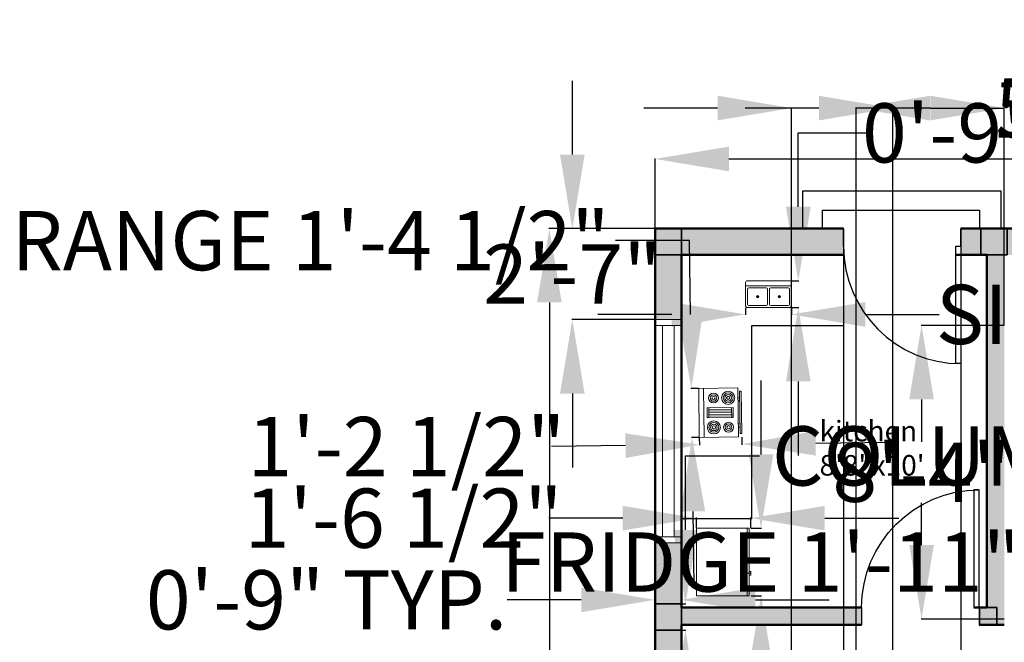
# Model space of a CAD drawing. Units: inches. Extents: x 25 to 82118, y 10 to 6494.
# Tile 2 of 9: x 40498 to 40833, y 3391 to 3603. Entities that reach past the tile are written whole.
import ezdxf

# ---------------------------------------------------------------- set-up
doc = ezdxf.new("R2010")
doc.units = ezdxf.units.IN
doc.header["$MEASUREMENT"] = 0
for name, color, linetype, lineweight in [('A-ANNO-DIMS', 2, 'Continuous', 18), ('A-AREA-IDEN', 7, 'Continuous', 25), ('A-DOOR', 3, 'Continuous', 25), ('A-EQPM', 8, 'Continuous', 18), ('A-FLOR-CASE', 8, 'Continuous', 25), ('A-FLOR-FIXT', 9, 'Continuous', 18), ('A-FLOR-STRS', 7, 'Continuous', 25), ('A-GLAZ', 4, 'Continuous', 18), ('A-WALL', 7, 'Continuous', 50)]:
    doc.layers.add(name, color=color, linetype=linetype, lineweight=lineweight)
doc.layers.add('A-COLS', color=30, linetype='Continuous', lineweight=35, true_color=0xf26722)
doc.layers.add('A-WALL-PATT', color=18, linetype='Continuous', lineweight=13, true_color=0x000000)
doc.styles.get("Standard").update_dxf_attribs({"font": 'arial.ttf'})
doc.dimstyles.get("Standard").update_dxf_attribs({"dimtxt": 20.18, "dimasz": 25.18, "dimexe": 0.18, "dimexo": 0.0625, "dimgap": 0.09, "dimtad": 0, "dimtih": 1, "dimtoh": 1, "dimdec": 0, "dimzin": 0, "dimdsep": 46, "dimlunit": 3, "dimtxsty": 'Standard', "dimcen": 0.09, "dimadec": 0, "dimazin": 0, "dimtfac": 1, "dimtdec": 0, "dimtofl": 0, "dimtmove": 0, "dimatfit": 3, "dimfxl": 1, "dimtolj": 1, "dimtzin": 0, "dimarcsym": 0})

# ---------------------------------------------------------------- blocks, each defined once
blk = doc.blocks.new('Sink-double - 36 in top')
for p, q in [((-18, -4), (18, -4)), ((-0.75, -18.5), (-0.75, -6.5)), ((0.75, -6.5), (0.75, -18.5))]:
    blk.add_line(p, q)
for points in [[(-16.5, 0), (16.5, 0)], [(-18, -19.5), (-18, -1.5)], [(-16.5, -18.5), (-16.5, -6.5)], [(-15.5, -5.5), (-1.75, -5.5)], [(1.75, -5.5), (15.5, -5.5)], [(16.5, -6.5), (16.5, -18.5)], [(18, -1.5), (18, -19.5)], [(16.5, -21), (-16.5, -21)], [(-1.75, -19.5), (-15.5, -19.5)], [(15.5, -19.5), (1.75, -19.5)]]:
    blk.add_lwpolyline(points)
for centre, radius in [((-8.5, -12.5), 1), ((-8.5, -12.5), 0.5), ((8.5, -12.5), 1), ((8.5, -12.5), 0.5)]:
    blk.add_circle(centre, radius)
for centre, radius, start, end in [((-16.5, -1.5), 1.5, 90, 180), ((16.5, -1.5), 1.5, 0, 90), ((-15.5, -6.5), 1, 90, 180), ((-1.75, -6.5), 1, 0, 90), ((1.75, -6.5), 1, 90, 180), ((15.5, -6.5), 1, 0, 90), ((-16.5, -19.5), 1.5, 180, 270), ((-15.5, -18.5), 1, 180, 270), ((-1.75, -18.5), 1, 270, 0), ((1.75, -18.5), 1, 180, 270), ((15.5, -18.5), 1, 270, 0), ((16.5, -19.5), 1.5, 270, 0)]:
    blk.add_arc(centre, radius, start, end)
blk = doc.blocks.new('Range-Oven - 30 in top')
for p, q in [((0, -3), (30, -3)), ((12, -6), (18, -6)), ((13, -20), (13, -6)), ((14, -6), (14, -20)), ((15, -20), (15, -6)), ((16, -6), (16, -20)), ((17, -20), (17, -6)), ((6, -24), (6, -25)), ((8, -25), (8, -24)), ((18, -20), (12, -20)), ((22, -25), (22, -24)), ((24, -24), (24, -25))]:
    blk.add_line(p, q)
for points in [[(0, -24), (0, 0), (30, 0), (30, -24)], [(12, -21), (12, -5), (18, -5), (18, -21)], [(2, -26), (2, -25), (28, -25), (28, -26)]]:
    blk.add_lwpolyline(points, close=True)
for centre, radius in [((6, -9), 4), ((6, -9), 3), ((24, -9), 3), ((6, -9), 2), ((6, -9), 1), ((24, -9), 2), ((24, -9), 1), ((6, -18), 3), ((6, -18), 2), ((6, -18), 1), ((24, -18), 4), ((24, -18), 3), ((24, -18), 2), ((24, -18), 1)]:
    blk.add_circle(centre, radius)
blk = doc.blocks.new('*U12')
for p, q in [((0, 0), (0, -6)), ((40, 0), (40, -6))]:
    blk.add_line(p, q)
blk.add_lwpolyline([(0, 0), (0, 40), (1.75, 40), (1.75, 0)], close=True)
blk.add_arc((0, 0), 40, 0, 90)
blk = doc.blocks.new('Refrigerator-2 door - 36 in top')
for p, q in [((0, -26.999999), (36, -26.999999)), ((11, -27.999999), (11, -28.999999)), ((11, -28.999999), (13, -28.999999)), ((12, -26.999999), (12, -28.999999)), ((13, -28.999999), (13, -27.999999))]:
    blk.add_line(p, q)
blk.add_lwpolyline([(0, -27.999999), (0, 0), (36, 0), (36, -27.999999)], close=True)
blk = doc.blocks.new('*D13')
at = {"layer": 'A-ANNO-DIMS', "color": 0, "lineweight": -2, "transparency": 16777216}
for p, q in [((40714.21, 3531.88), (40714.21, 3555.71)), ((40739.39, 3555.53), (40877, 3555.53)), ((41049.03, 3555.53), (40911.42, 3555.53)), ((41074.21, 3531.88), (41074.21, 3555.71))]:
    blk.add_line(p, q, dxfattribs=at)
at = {"layer": 'A-ANNO-DIMS', "color": 0, "transparency": 16777216}
for points in [[(40739.39, 3559.72), (40739.39, 3551.33), (40714.21, 3555.53)], [(41049.03, 3559.72), (41049.03, 3551.33), (41074.21, 3555.53)]]:
    blk.add_solid(points, dxfattribs=at)
at = {"layer": 'Defpoints', "color": 0, "transparency": 16777216}
for p in [(41074.21, 3555.53), (40714.21, 3531.82), (41074.21, 3531.82)]:
    blk.add_point(p, dxfattribs=at)
at = {"layer": 'A-ANNO-DIMS', "color": 0, "transparency": 16777216, "insert": (40894.21, 3555.53), "char_height": 20.18, "attachment_point": 5}
blk.add_mtext("\\A1;30'", dxfattribs=at)
blk = doc.blocks.new('*D14')
at = {"layer": 'A-ANNO-DIMS', "color": 0, "lineweight": -2, "transparency": 16777216}
for p, q in [((40714.15, 3531.82), (40678.01, 3531.82)), ((40678.19, 3506.64), (40678.19, 3350.2)), ((40678.19, 3172.97), (40678.19, 3329.4)), ((40714.15, 3147.79), (40678.01, 3147.79))]:
    blk.add_line(p, q, dxfattribs=at)
at = {"layer": 'A-ANNO-DIMS', "color": 0, "transparency": 16777216}
for points in [[(40673.99, 3506.64), (40682.39, 3506.64), (40678.19, 3531.82)], [(40673.99, 3172.97), (40682.39, 3172.97), (40678.19, 3147.79)]]:
    blk.add_solid(points, dxfattribs=at)
at = {"layer": 'Defpoints', "color": 0, "transparency": 16777216}
for p in [(40714.21, 3531.82), (40678.19, 3147.79), (40714.21, 3147.79)]:
    blk.add_point(p, dxfattribs=at)
at = {"layer": 'A-ANNO-DIMS', "color": 0, "transparency": 16777216, "insert": (40678.19, 3339.8), "char_height": 20.18, "attachment_point": 5}
blk.add_mtext("\\A1;32'", dxfattribs=at)
blk = doc.blocks.new('WIN-72IN-9W')
for p, q in [((9, 76), (0, 76)), ((9, 74), (0, 74)), ((2.5, 74), (2.5, 2)), ((6.5, 74), (6.5, 2)), ((9, 2), (0, 2)), ((9, 0), (0, 0))]:
    blk.add_line(p, q)
blk = doc.blocks.new('COL-9X9')
h = blk.add_hatch(color=256)
h.dxf.hatch_style = 1
h.paths.add_polyline_path([(9, 9), (0, 9), (0, 0), (9, 0)])
blk.add_lwpolyline([(0, 0), (9, 0), (9, 9), (0, 9)], close=True)
blk = doc.blocks.new('POST-INTERIOR-6IN')
h = blk.add_hatch(color=256)
h.dxf.hatch_style = 1
h.paths.add_polyline_path([(6, 5.8), (0, 5.8), (0, 0), (6, 0)])
blk.add_lwpolyline([(6, 5.8), (0, 5.8), (0, 0), (6, 0)], close=True)
blk = doc.blocks.new('*D25')
at = {"layer": 'A-ANNO-DIMS', "color": 0, "lineweight": -2, "transparency": 16777216}
for p, q in [((40724.56, 3429.21), (40724.56, 3454.39)), ((40724.56, 3454.39), (40749.74, 3454.39)), ((40723.27, 3404.03), (40724.74, 3404.03)), ((40723.27, 3395.03), (40724.74, 3395.03)), ((40724.56, 3369.85), (40724.56, 3344.67))]:
    blk.add_line(p, q, dxfattribs=at)
at = {"layer": 'A-ANNO-DIMS', "color": 0, "transparency": 16777216}
for points in [[(40720.36, 3429.21), (40728.76, 3429.21), (40724.56, 3404.03)], [(40720.36, 3369.85), (40728.76, 3369.85), (40724.56, 3395.03)]]:
    blk.add_solid(points, dxfattribs=at)
at = {"layer": 'Defpoints', "color": 0, "transparency": 16777216}
for p in [(40723.21, 3404.03), (40724.56, 3404.03), (40723.21, 3395.03)]:
    blk.add_point(p, dxfattribs=at)
at = {"layer": 'A-ANNO-DIMS', "color": 0, "transparency": 16777216, "insert": (40876.22, 3454.39), "char_height": 20.18, "attachment_point": 5}
blk.add_mtext('\\A1;COLUMN 0\'-9" TYP.', dxfattribs=at)
blk = doc.blocks.new('*D26')
at = {"layer": 'A-ANNO-DIMS', "color": 0, "lineweight": -2, "transparency": 16777216}
for p, q in [((40714.21, 3404.09), (40714.21, 3405.56)), ((40723.21, 3404.09), (40723.21, 3405.56)), ((40689.03, 3405.38), (40663.85, 3405.38)), ((40748.39, 3405.38), (40773.57, 3405.38))]:
    blk.add_line(p, q, dxfattribs=at)
at = {"layer": 'A-ANNO-DIMS', "color": 0, "transparency": 16777216}
for points in [[(40689.03, 3409.57), (40689.03, 3401.18), (40714.21, 3405.38)], [(40748.39, 3409.57), (40748.39, 3401.18), (40723.21, 3405.38)]]:
    blk.add_solid(points, dxfattribs=at)
at = {"layer": 'Defpoints', "color": 0, "transparency": 16777216}
for p in [(40714.21, 3405.38), (40714.21, 3404.03), (40723.21, 3404.03)]:
    blk.add_point(p, dxfattribs=at)
at = {"layer": 'A-ANNO-DIMS', "color": 0, "transparency": 16777216, "insert": (40602.26, 3405.38), "char_height": 20.18, "attachment_point": 5}
blk.add_mtext('\\A1;0\'-9" TYP.', dxfattribs=at)
blk = doc.blocks.new('*D37')
at = {"layer": 'A-ANNO-DIMS', "color": 0, "lineweight": -2, "transparency": 16777216}
for p, q in [((40745.04, 3504.86), (40745.04, 3502.4)), ((40760.67, 3504.86), (40760.67, 3502.4)), ((40719.86, 3502.58), (40694.68, 3502.58)), ((40785.85, 3502.58), (40811.03, 3502.58))]:
    blk.add_line(p, q, dxfattribs=at)
at = {"layer": 'A-ANNO-DIMS', "color": 0, "transparency": 16777216}
for points in [[(40719.86, 3506.78), (40719.86, 3498.38), (40745.04, 3502.58)], [(40785.85, 3506.78), (40785.85, 3498.38), (40760.67, 3502.58)]]:
    blk.add_solid(points, dxfattribs=at)
at = {"layer": 'Defpoints', "color": 0, "transparency": 16777216}
for p in [(40745.04, 3504.92), (40760.67, 3504.92), (40760.67, 3502.58)]:
    blk.add_point(p, dxfattribs=at)
at = {"layer": 'A-ANNO-DIMS', "color": 0, "transparency": 16777216, "insert": (40898.22, 3502.58), "char_height": 20.18, "attachment_point": 5}
blk.add_mtext('\\A1;SINK 1\'-3 1/2"', dxfattribs=at)
blk = doc.blocks.new('*D38')
at = {"layer": 'A-ANNO-DIMS', "color": 0, "lineweight": -2, "transparency": 16777216}
for p, q in [((40763.01, 3539.22), (40763.01, 3564.4)), ((40763.01, 3564.4), (40788.19, 3564.4)), ((40760.73, 3514.04), (40763.19, 3514.04)), ((40760.73, 3504.92), (40763.19, 3504.92)), ((40763.01, 3479.74), (40763.01, 3454.56))]:
    blk.add_line(p, q, dxfattribs=at)
at = {"layer": 'A-ANNO-DIMS', "color": 0, "transparency": 16777216}
for points in [[(40758.81, 3539.22), (40767.21, 3539.22), (40763.01, 3514.04)], [(40758.81, 3479.74), (40767.21, 3479.74), (40763.01, 3504.92)]]:
    blk.add_solid(points, dxfattribs=at)
at = {"layer": 'Defpoints', "color": 0, "transparency": 16777216}
for p in [(40760.67, 3514.04), (40763.01, 3514.04), (40760.67, 3504.92)]:
    blk.add_point(p, dxfattribs=at)
at = {"layer": 'A-ANNO-DIMS', "color": 0, "transparency": 16777216, "insert": (40815.1, 3564.4), "char_height": 20.18, "attachment_point": 5}
blk.add_mtext('\\A1;0\'-9"', dxfattribs=at)
blk = doc.blocks.new('*D39')
at = {"layer": 'A-ANNO-DIMS', "color": 0, "lineweight": -2, "transparency": 16777216}
for p, q in [((40725.94, 3527.71), (40700.76, 3527.71)), ((40726.26, 3502.53), (40725.94, 3527.71)), ((40729.01, 3477.38), (40726.39, 3477.35)), ((40729.22, 3460.71), (40726.6, 3460.68)), ((40727.1, 3435.5), (40727.41, 3410.32))]:
    blk.add_line(p, q, dxfattribs=at)
at = {"layer": 'A-ANNO-DIMS', "color": 0, "transparency": 16777216}
for points in [[(40730.45, 3502.58), (40722.06, 3502.48), (40726.57, 3477.35)], [(40731.29, 3435.55), (40722.9, 3435.45), (40726.78, 3460.68)]]:
    blk.add_solid(points, dxfattribs=at)
at = {"layer": 'Defpoints', "color": 0, "transparency": 16777216}
for p in [(40726.57, 3477.35), (40729.07, 3477.38), (40729.28, 3460.71)]:
    blk.add_point(p, dxfattribs=at)
at = {"layer": 'A-ANNO-DIMS', "color": 0, "transparency": 16777216, "insert": (40596.82, 3527.71), "char_height": 20.18, "attachment_point": 5}
blk.add_mtext('\\A1;RANGE 1\'-4 1/2"', dxfattribs=at)
blk = doc.blocks.new('*D40')
at = {"layer": 'A-ANNO-DIMS', "color": 0, "lineweight": -2, "transparency": 16777216}
for p, q in [((40729.28, 3460.65), (40729.32, 3458.03)), ((40743.73, 3460.83), (40743.76, 3458.21)), ((40704.14, 3457.89), (40678.96, 3457.58)), ((40768.94, 3458.71), (40794.12, 3459.02))]:
    blk.add_line(p, q, dxfattribs=at)
at = {"layer": 'A-ANNO-DIMS', "color": 0, "transparency": 16777216}
for points in [[(40768.89, 3462.9), (40768.99, 3454.51), (40743.76, 3458.39)], [(40704.08, 3462.09), (40704.19, 3453.7), (40729.31, 3458.21)]]:
    blk.add_solid(points, dxfattribs=at)
at = {"layer": 'Defpoints', "color": 0, "transparency": 16777216}
for p in [(40729.28, 3460.71), (40743.73, 3460.89), (40729.31, 3458.21)]:
    blk.add_point(p, dxfattribs=at)
at = {"layer": 'A-ANNO-DIMS', "color": 0, "transparency": 16777216, "insert": (40629.48, 3457.58), "char_height": 20.18, "attachment_point": 5}
blk.add_mtext('\\A1;1\'-2 1/2"', dxfattribs=at)
blk = doc.blocks.new('*D51')
at = {"layer": 'A-ANNO-DIMS', "color": 0, "lineweight": -2, "transparency": 16777216}
for p, q in [((40750.31, 3454.92), (40750.31, 3480.1)), ((40746.92, 3429.74), (40750.49, 3429.74)), ((40746.92, 3406.76), (40750.49, 3406.76)), ((40750.31, 3381.58), (40750.31, 3356.4))]:
    blk.add_line(p, q, dxfattribs=at)
at = {"layer": 'A-ANNO-DIMS', "color": 0, "transparency": 16777216}
for points in [[(40746.11, 3454.92), (40754.5, 3454.92), (40750.31, 3429.74)], [(40746.11, 3381.58), (40754.5, 3381.58), (40750.31, 3406.76)]]:
    blk.add_solid(points, dxfattribs=at)
at = {"layer": 'Defpoints', "color": 0, "transparency": 16777216}
for p in [(40746.86, 3429.74), (40750.31, 3429.74), (40746.86, 3406.76)]:
    blk.add_point(p, dxfattribs=at)
at = {"layer": 'A-ANNO-DIMS', "color": 0, "transparency": 16777216, "insert": (40750.31, 3418.25), "char_height": 20.18, "attachment_point": 5}
blk.add_mtext('\\A1;FRIDGE 1\'-11"', dxfattribs=at)
blk = doc.blocks.new('*D52')
at = {"layer": 'A-ANNO-DIMS', "color": 0, "lineweight": -2, "transparency": 16777216}
for p, q in [((40703.17, 3433.19), (40677.99, 3433.19)), ((40728.35, 3429.8), (40728.35, 3433.37)), ((40746.86, 3429.8), (40746.86, 3433.37)), ((40772.04, 3433.19), (40797.22, 3433.19))]:
    blk.add_line(p, q, dxfattribs=at)
at = {"layer": 'A-ANNO-DIMS', "color": 0, "transparency": 16777216}
for points in [[(40703.17, 3437.39), (40703.17, 3428.99), (40728.35, 3433.19)], [(40772.04, 3437.39), (40772.04, 3428.99), (40746.86, 3433.19)]]:
    blk.add_solid(points, dxfattribs=at)
at = {"layer": 'Defpoints', "color": 0, "transparency": 16777216}
for p in [(40728.35, 3433.19), (40728.35, 3429.74), (40746.86, 3429.74)]:
    blk.add_point(p, dxfattribs=at)
at = {"layer": 'A-ANNO-DIMS', "color": 0, "transparency": 16777216, "insert": (40628.52, 3433.19), "char_height": 20.18, "attachment_point": 5}
blk.add_mtext('\\A1;1\'-6 1/2"', dxfattribs=at)
blk = doc.blocks.new('*D53')
at = {"layer": 'A-ANNO-DIMS', "color": 0, "lineweight": -2, "transparency": 16777216}
for p, q in [((40808.03, 3572.85), (40782.85, 3572.85)), ((40833.21, 3498.88), (40833.21, 3573.03)), ((40903.21, 3498.88), (40903.21, 3573.03)), ((40928.39, 3572.85), (40953.57, 3572.85))]:
    blk.add_line(p, q, dxfattribs=at)
at = {"layer": 'A-ANNO-DIMS', "color": 0, "transparency": 16777216}
for points in [[(40808.03, 3577.05), (40808.03, 3568.66), (40833.21, 3572.85)], [(40928.39, 3577.05), (40928.39, 3568.66), (40903.21, 3572.85)]]:
    blk.add_solid(points, dxfattribs=at)
at = {"layer": 'Defpoints', "color": 0, "transparency": 16777216}
for p in [(40903.21, 3572.85), (40833.21, 3498.82), (40903.21, 3498.82)]:
    blk.add_point(p, dxfattribs=at)
at = {"layer": 'A-ANNO-DIMS', "color": 0, "transparency": 16777216, "insert": (40868.21, 3572.85), "char_height": 20.18, "attachment_point": 5}
blk.add_mtext('\\A1;5\'-10"', dxfattribs=at)
blk = doc.blocks.new('*D54')
at = {"layer": 'A-ANNO-DIMS', "color": 0, "lineweight": -2, "transparency": 16777216}
for p, q in [((40833.15, 3498.82), (40804.83, 3498.82)), ((40805.01, 3473.64), (40805.01, 3459.21)), ((40805.01, 3424), (40805.01, 3438.43)), ((40833.15, 3398.82), (40804.83, 3398.82))]:
    blk.add_line(p, q, dxfattribs=at)
at = {"layer": 'A-ANNO-DIMS', "color": 0, "transparency": 16777216}
for points in [[(40800.81, 3473.64), (40809.21, 3473.64), (40805.01, 3498.82)], [(40800.81, 3424), (40809.21, 3424), (40805.01, 3398.82)]]:
    blk.add_solid(points, dxfattribs=at)
at = {"layer": 'Defpoints', "color": 0, "transparency": 16777216}
for p in [(40805.01, 3498.82), (40833.21, 3498.82), (40833.21, 3398.82)]:
    blk.add_point(p, dxfattribs=at)
at = {"layer": 'A-ANNO-DIMS', "color": 0, "transparency": 16777216, "insert": (40805.01, 3448.82), "char_height": 20.18, "attachment_point": 5}
blk.add_mtext('\\A1;8\'-4"', dxfattribs=at)
blk = doc.blocks.new('*D56')
at = {"layer": 'A-ANNO-DIMS', "color": 0, "lineweight": -2, "transparency": 16777216}
for p, q in [((40778.43, 3531.76), (40778.43, 3119.41)), ((40818.43, 3531.76), (40818.43, 3119.41)), ((40753.25, 3119.59), (40728.07, 3119.59)), ((40843.61, 3119.59), (40868.79, 3119.59))]:
    blk.add_line(p, q, dxfattribs=at)
at = {"layer": 'A-ANNO-DIMS', "color": 0, "transparency": 16777216}
for points in [[(40753.25, 3123.78), (40753.25, 3115.39), (40778.43, 3119.59)], [(40843.61, 3123.78), (40843.61, 3115.39), (40818.43, 3119.59)]]:
    blk.add_solid(points, dxfattribs=at)
at = {"layer": 'Defpoints', "color": 0, "transparency": 16777216}
for p in [(40778.43, 3531.82), (40818.43, 3531.82), (40818.43, 3119.59)]:
    blk.add_point(p, dxfattribs=at)
at = {"layer": 'A-ANNO-DIMS', "color": 0, "transparency": 16777216, "insert": (40895.69, 3119.59), "char_height": 20.18, "attachment_point": 5}
blk.add_mtext('\\A1;3\'-4"', dxfattribs=at)
blk = doc.blocks.new('*D57')
at = {"layer": 'A-ANNO-DIMS', "color": 0, "lineweight": -2, "transparency": 16777216}
for p, q in [((40714.21, 3531.76), (40714.21, 3119.41)), ((40778.43, 3531.76), (40778.43, 3119.41)), ((40689.03, 3119.59), (40663.85, 3119.59)), ((40803.61, 3119.59), (40828.79, 3119.59))]:
    blk.add_line(p, q, dxfattribs=at)
at = {"layer": 'A-ANNO-DIMS', "color": 0, "transparency": 16777216}
for points in [[(40689.03, 3123.78), (40689.03, 3115.39), (40714.21, 3119.59)], [(40803.61, 3123.78), (40803.61, 3115.39), (40778.43, 3119.59)]]:
    blk.add_solid(points, dxfattribs=at)
at = {"layer": 'Defpoints', "color": 0, "transparency": 16777216}
for p in [(40714.21, 3531.82), (40778.43, 3531.82), (40778.43, 3119.59)]:
    blk.add_point(p, dxfattribs=at)
at = {"layer": 'A-ANNO-DIMS', "color": 0, "transparency": 16777216, "insert": (40746.32, 3119.59), "char_height": 20.18, "attachment_point": 5}
blk.add_mtext('\\A1;5\'-4"', dxfattribs=at)
blk = doc.blocks.new('*D58')
at = {"layer": 'A-ANNO-DIMS', "color": 0, "lineweight": -2, "transparency": 16777216}
for p, q in [((40735.53, 3572.85), (40710.35, 3572.85)), ((40760.71, 3246.88), (40760.71, 3573.03)), ((40782.73, 3246.88), (40782.73, 3573.03)), ((40807.91, 3572.85), (40833.09, 3572.85))]:
    blk.add_line(p, q, dxfattribs=at)
at = {"layer": 'A-ANNO-DIMS', "color": 0, "transparency": 16777216}
for points in [[(40735.53, 3577.05), (40735.53, 3568.66), (40760.71, 3572.85)], [(40807.91, 3577.05), (40807.91, 3568.66), (40782.73, 3572.85)]]:
    blk.add_solid(points, dxfattribs=at)
at = {"layer": 'Defpoints', "color": 0, "transparency": 16777216}
for p in [(40782.73, 3572.85), (40760.71, 3246.82), (40782.73, 3246.82)]:
    blk.add_point(p, dxfattribs=at)
at = {"layer": 'A-ANNO-DIMS', "color": 0, "transparency": 16777216, "insert": (40866.89, 3572.85), "char_height": 20.18, "attachment_point": 5}
blk.add_mtext('\\A1;1\'-10"', dxfattribs=at)
blk = doc.blocks.new('*D63')
at = {"layer": 'A-ANNO-DIMS', "color": 0, "lineweight": -2, "transparency": 16777216}
for p, q in [((40686.01, 3557), (40686.01, 3582.18)), ((40714.15, 3531.82), (40685.83, 3531.82)), ((40714.15, 3500.82), (40685.83, 3500.82)), ((40686.01, 3475.64), (40686.01, 3450.46))]:
    blk.add_line(p, q, dxfattribs=at)
at = {"layer": 'A-ANNO-DIMS', "color": 0, "transparency": 16777216}
for points in [[(40681.81, 3557), (40690.21, 3557), (40686.01, 3531.82)], [(40681.81, 3475.64), (40690.21, 3475.64), (40686.01, 3500.82)]]:
    blk.add_solid(points, dxfattribs=at)
at = {"layer": 'Defpoints', "color": 0, "transparency": 16777216}
for p in [(40686.01, 3531.82), (40714.21, 3531.82), (40714.21, 3500.82)]:
    blk.add_point(p, dxfattribs=at)
at = {"layer": 'A-ANNO-DIMS', "color": 0, "transparency": 16777216, "insert": (40686.01, 3516.32), "char_height": 20.18, "attachment_point": 5}
blk.add_mtext('\\A1;2\'-7"', dxfattribs=at)
blk = doc.blocks.new('*D67')
at = {"layer": 'A-ANNO-DIMS', "color": 0, "lineweight": -2, "transparency": 16777216}
for p, q in [((40770.03, 3572.85), (40744.85, 3572.85)), ((40795.21, 3156.88), (40795.21, 3573.03)), ((40838.63, 3156.88), (40838.63, 3573.03)), ((40863.81, 3572.85), (40888.99, 3572.85))]:
    blk.add_line(p, q, dxfattribs=at)
at = {"layer": 'A-ANNO-DIMS', "color": 0, "transparency": 16777216}
for points in [[(40770.03, 3577.05), (40770.03, 3568.66), (40795.21, 3572.85)], [(40863.81, 3577.05), (40863.81, 3568.66), (40838.63, 3572.85)]]:
    blk.add_solid(points, dxfattribs=at)
at = {"layer": 'Defpoints', "color": 0, "transparency": 16777216}
for p in [(40838.63, 3572.85), (40795.21, 3156.82), (40838.63, 3156.82)]:
    blk.add_point(p, dxfattribs=at)
at = {"layer": 'A-ANNO-DIMS', "color": 0, "transparency": 16777216, "insert": (40939.41, 3572.85), "char_height": 20.18, "attachment_point": 5}
blk.add_mtext('\\A1;3\'-7 1/2"', dxfattribs=at)

msp = doc.modelspace()

# ---------------------------------------------------------------- hatches: boundary and pattern name
at = {"layer": 'A-WALL-PATT'}
h = msp.add_hatch(color=256, dxfattribs=at)
h.dxf.hatch_style = 1
h.paths.add_polyline_path([(40778.43, 3531.82), (40723.21, 3531.82), (40723.21, 3522.82), (40778.54, 3522.82, -0.01877), (40778.43, 3525.82)])
h.paths.add_polyline_path([(40723.21, 3522.82), (40714.21, 3522.82), (40714.21, 3500.82), (40723.21, 3500.82)])
h.paths.add_polyline_path([(40723.21, 3424.82), (40714.21, 3424.82), (40714.21, 3404.03), (40723.21, 3404.03)])
h.paths.add_polyline_path([(40723.21, 3395.03), (40714.21, 3395.03), (40714.21, 3386.82), (40723.21, 3386.82)])
h.paths.add_polyline_path([(40901.65, 3531.82), (40834.16, 3531.82), (40834.16, 3522.82), (40901.65, 3522.82)])
h.paths.add_polyline_path([(40825.16, 3531.82), (40818.43, 3531.82), (40818.43, 3525.82), (40818.43, 3522.82), (40825.16, 3522.82)])
h.paths.add_polyline_path([(40961.21, 3531.82), (40910.65, 3531.82), (40910.65, 3522.82), (40961.21, 3522.82)])
h.paths.add_polyline_path([(41065.21, 3531.82), (41013.21, 3531.82), (41013.21, 3522.82), (41065.21, 3522.82)])
h.paths.add_polyline_path([(41074.21, 3522.82), (41065.21, 3522.82), (41065.21, 3506.52), (41074.21, 3506.52)])
h.paths.add_polyline_path([(41074.21, 3430.52), (41065.21, 3430.52), (41065.21, 3428.74), (41065.21, 3380.62), (41074.21, 3380.62)])
h.paths.add_polyline_path([(41074.21, 3371.62), (41065.21, 3371.62), (41065.21, 3355.41), (41074.21, 3355.41)])
h.paths.add_polyline_path([(41065.36, 3378.82), (40909.21, 3378.82), (40909.21, 3382.1), (40903.21, 3382.1), (40903.21, 3372.82), (41065.36, 3372.82)])
h.paths.add_polyline_path([(40933.21, 3372.82), (40927.21, 3372.82), (40927.21, 3282.62), (40933.21, 3282.62)])
h.paths.add_polyline_path([(41074.21, 3279.41), (41065.21, 3279.41), (41065.21, 3240.82), (41074.21, 3240.82)])
h.paths.add_polyline_path([(41065.21, 3246.82), (41052.05, 3246.82), (41052.05, 3240.82), (41065.21, 3240.82)])
h.paths.add_polyline_path([(40985.75, 3202.89), (41023.1, 3202.89), (41023.1, 3229.01), (40985.75, 3229.01)], flags=9)
h.paths.add_polyline_path([(40960.75, 3302.54), (40998.1, 3302.54), (40998.1, 3328.66), (40960.75, 3328.66)], flags=9)
h = msp.add_hatch(color=256, dxfattribs=at)
h.dxf.hatch_style = 1
h.paths.add_polyline_path([(40784.59, 3402.82), (40723.21, 3402.82), (40723.21, 3396.82), (40784.59, 3396.82)])
h.paths.add_polyline_path([(40833.21, 3522.82), (40827.21, 3522.82), (40827.21, 3402.75), (40830.71, 3402.75), (40830.71, 3396.82), (40833.21, 3396.82)])
h.paths.add_polyline_path([(40767.21, 3280.82), (40723.21, 3280.82), (40723.21, 3274.82), (40767.21, 3274.82)])
h.paths.add_polyline_path([(40723.21, 3288.82), (40714.21, 3288.82), (40714.21, 3283), (40723.21, 3283)])

# ---------------------------------------------------------------- linework, layer by layer
at = {"layer": 'A-FLOR-CASE'}
for p, q in [((40778.54, 3498.82), (40778.54, 3522.82)), ((40747.21, 3432.97), (40747.21, 3498.82)), ((40747.21, 3498.82), (40778.54, 3498.82)), ((40747.21, 3432.97), (40723.21, 3432.97))]:
    msp.add_line(p, q, dxfattribs=at)
at = {"layer": 'A-FLOR-STRS'}
for p, q in [((40764.61, 3531.82), (40764.61, 3544.65)), ((40764.61, 3544.65), (40832.08, 3544.65)), ((40832.08, 3544.65), (40832.08, 3531.82)), ((40771.24, 3531.82), (40771.24, 3538.04)), ((40771.24, 3538.04), (40824.76, 3538.04)), ((40824.76, 3538.04), (40824.76, 3531.82))]:
    msp.add_line(p, q, dxfattribs=at)
at = {"layer": 'A-WALL'}
for p, q in [((40714.21, 3147.82), (40714.21, 3531.82)), ((40714.21, 3531.82), (40778.43, 3531.82)), ((40818.43, 3531.82), (41074.21, 3531.82)), ((40723.21, 3522.82), (40778.54, 3522.82)), ((40723.21, 3402.82), (40723.21, 3522.82)), ((40816.68, 3522.82), (40827.21, 3522.82)), ((40827.21, 3402.82), (40827.21, 3522.82)), ((40723.21, 3402.82), (40784.59, 3402.82)), ((40822.84, 3402.82), (40827.21, 3402.82)), ((40723.21, 3396.82), (40784.59, 3396.82)), ((40723.21, 3280.82), (40723.21, 3396.82)), ((40824.59, 3396.82), (40833.21, 3396.82))]:
    msp.add_line(p, q, dxfattribs=at)

# ---------------------------------------------------------------- block references
at = {"layer": 'A-COLS'}
for p, rotation in [((40723.21, 3522.82), 89.99999999991604), ((40834.16, 3522.82), 89.99999999996236), ((40723.21, 3395.03), 89.99999999991604)]:
    msp.add_blockref('COL-9X9', p, dxfattribs=dict(at, rotation=rotation))
msp.add_blockref('POST-INTERIOR-6IN', (40824.71, 3396.95), dxfattribs=at)
at = {"layer": 'A-DOOR', "rotation": 180}
msp.add_blockref('*U12', (40818.43, 3525.82), dxfattribs=at)
at = {"layer": 'A-DOOR', "xscale": -1}
msp.add_blockref('*U12', (40824.59, 3402.82), dxfattribs=at)
at = {"layer": 'A-EQPM'}
for name, p, xscale, yscale, zscale, rotation in [('Range-Oven - 30 in top', (40729.28, 3460.71), 0.5557370614235423, 0.5557370614235423, 0.5557370614235423, 90.71973134519538), ('Refrigerator-2 door - 36 in top', (40728.35, 3406.76), 0.6383624943621964, 0.6383624943621964, 0.6383624943621964, 90)]:
    msp.add_blockref(name, p, dxfattribs=dict(at, xscale=xscale, yscale=yscale, zscale=zscale, rotation=rotation))
at = {"layer": 'A-FLOR-FIXT', "xscale": 0.4341249891135496, "yscale": 0.4341249891135496, "zscale": 0.4341249891135496}
msp.add_blockref('Sink-double - 36 in top', (40752.85, 3514.04), dxfattribs=at)
at = {"layer": 'A-GLAZ'}
msp.add_blockref('WIN-72IN-9W', (40714.21, 3424.82), dxfattribs=at)

# ---------------------------------------------------------------- texts
at = {"layer": 'A-AREA-IDEN', "insert": (40770.24, 3466.36), "char_height": 7, "attachment_point": 1}
msp.add_mtext_dynamic_manual_height_columns('kitchen\\P8\'8"x10\'', width=132.9687, gutter_width=1, heights=[0], dxfattribs=at)

# ---------------------------------------------------------------- dimensions: what is measured, and where the dimension line sits
at = {"layer": 'A-ANNO-DIMS'}
for base, p1, p2, override, picture, middle in [((40838.63, 3572.85), (40795.21, 3156.82), (40838.63, 3156.82), {"dimdec": 1, "dimlfac": 1, "dimrnd": 0, "dimzin": 1, "dimdsep": 46, "dimlunit": 4, "dimfrac": 2}, '*D67', (40939.41, 3572.85)), ((40782.73, 3572.85), (40760.71, 3246.82), (40782.73, 3246.82), {"dimdec": 1, "dimlfac": 1, "dimrnd": 0, "dimzin": 1, "dimdsep": 46, "dimlunit": 4, "dimfrac": 2}, '*D58', (40866.89, 3572.85)), ((40903.21, 3572.85), (40833.21, 3498.82), (40903.21, 3498.82), {"dimdec": 1, "dimlfac": 1, "dimrnd": 0, "dimzin": 1, "dimdsep": 46, "dimlunit": 4, "dimfrac": 2}, '*D53', (40868.21, 3572.85)), ((41074.21, 3555.53), (40714.21, 3531.82), (41074.21, 3531.82), {"dimclrd": 0, "dimclre": 0, "dimclrt": 0}, '*D13', (40894.21, 3555.53)), ((40778.43, 3119.59), (40714.21, 3531.82), (40778.43, 3531.82), {"dimdec": 1, "dimlfac": 1, "dimrnd": 0, "dimzin": 1, "dimdsep": 46, "dimlunit": 4, "dimfrac": 2}, '*D57', (40746.32, 3119.59)), ((40818.43, 3119.59), (40778.43, 3531.82), (40818.43, 3531.82), {"dimdec": 1, "dimlfac": 1, "dimrnd": 0, "dimzin": 1, "dimdsep": 46, "dimlunit": 4, "dimfrac": 2}, '*D56', (40895.69, 3119.59))]:
    dim = msp.add_linear_dim(base=base, p1=p1, p2=p2, dimstyle='Standard', override=override, dxfattribs=at)
    dim.commit()
    dim.dimension.update_dxf_attribs({"geometry": picture, "text_midpoint": middle})
for base, p1, p2, angle, override, picture, middle in [((40686.01, 3531.82), (40714.21, 3500.82), (40714.21, 3531.82), 90, {"dimdec": 1, "dimlfac": 1, "dimrnd": 0, "dimzin": 1, "dimdsep": 46, "dimlunit": 4, "dimfrac": 2}, '*D63', (40686.01, 3516.32)), ((40763.01, 3514.04), (40760.67, 3504.92), (40760.67, 3514.04), 90, {"dimdec": 1, "dimlfac": 1, "dimrnd": 0, "dimzin": 1, "dimdsep": 46, "dimlunit": 4, "dimfrac": 2}, '*D38', (40815.1, 3564.4)), ((40678.19, 3147.79), (40714.21, 3531.82), (40714.21, 3147.79), 90, {"dimclrd": 0, "dimclre": 0, "dimclrt": 0}, '*D14', (40678.19, 3339.8)), ((40805.01, 3498.82), (40833.21, 3398.82), (40833.21, 3498.82), 90, {"dimdec": 1, "dimlfac": 1, "dimrnd": 0, "dimzin": 1, "dimdsep": 46, "dimlunit": 4, "dimfrac": 2}, '*D54', (40805.01, 3448.82)), ((40729.3138, 3458.2097), (40743.7304, 3460.8918), (40729.2824, 3460.7103), 180.7197, {"dimdec": 1, "dimlfac": 1, "dimrnd": 0, "dimzin": 1, "dimdsep": 46, "dimlunit": 4, "dimfrac": 2}, '*D40', (40629.4846, 3457.5771)), ((40728.35, 3433.19), (40746.86, 3429.74), (40728.35, 3429.74), 180, {"dimdec": 1, "dimlfac": 1, "dimrnd": 0, "dimzin": 1, "dimdsep": 46, "dimlunit": 4, "dimfrac": 2}, '*D52', (40628.52, 3433.19))]:
    dim = msp.add_linear_dim(base=base, p1=p1, p2=p2, angle=angle, dimstyle='Standard', override=override, dxfattribs=at)
    dim.commit()
    dim.dimension.update_dxf_attribs({"geometry": picture, "text_midpoint": middle})
for base, p1, p2, angle, text, picture, middle in [((40726.57, 3477.35), (40729.28, 3460.71), (40729.07, 3477.38), 90.7197, 'RANGE <>', '*D39', (40596.82, 3527.71)), ((40724.56, 3404.03), (40723.21, 3395.03), (40723.21, 3404.03), 90, 'COLUMN <> TYP.', '*D25', (40876.22, 3454.39)), ((40750.31, 3429.74), (40746.86, 3406.76), (40746.86, 3429.74), 90, 'FRIDGE <>', '*D51', (40750.31, 3418.25)), ((40714.21, 3405.38), (40723.21, 3404.03), (40714.21, 3404.03), 180, '<> TYP.', '*D26', (40602.26, 3405.38))]:
    dim = msp.add_linear_dim(base=base, p1=p1, p2=p2, angle=angle, text=text, dimstyle='Standard', override={"dimdec": 1, "dimlfac": 1, "dimrnd": 0, "dimzin": 1, "dimdsep": 46, "dimlunit": 4, "dimfrac": 2}, dxfattribs=at)
    dim.commit()
    dim.dimension.update_dxf_attribs({"geometry": picture, "text_midpoint": middle})
dim = msp.add_linear_dim(base=(40760.67, 3502.58), p1=(40745.04, 3504.92), p2=(40760.67, 3504.92), text='SINK <>', dimstyle='Standard', override={"dimdec": 1, "dimlfac": 1, "dimrnd": 0, "dimzin": 1, "dimdsep": 46, "dimlunit": 4, "dimfrac": 2}, dxfattribs=at)
dim.commit()
dim.dimension.update_dxf_attribs({"geometry": '*D37', "text_midpoint": (40898.22, 3502.58)})

doc.saveas('drawing.dxf')
